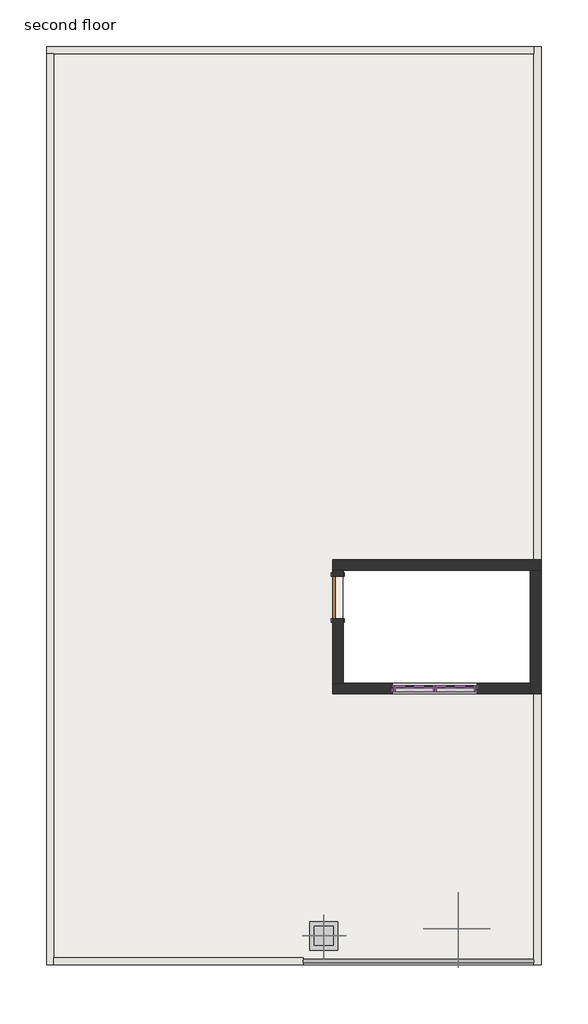
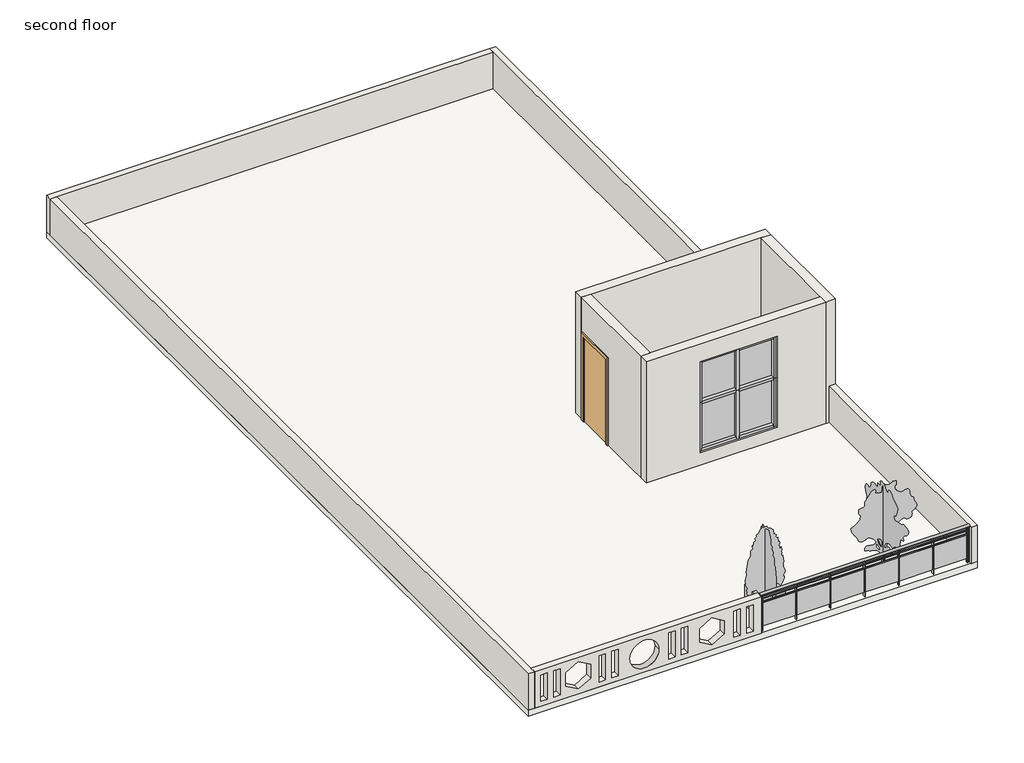
# One storey, incomplete: 12 members, 9 walls, 4 plates, 3 geographic elements, 1 door, 1 railing, 1 slab.
"""IFC4 building model written with IfcOpenShell, lengths in millimetres."""

from ifc_helpers import new_model, si_unit, point, frame, frame_2d, origin, place, context, project, spatial, polyline, circle_curve, ellipse_curve, trimmed, segment, composite_curve, outline, extrude, faceted_brep, transform, mapped, element, save
from ifc_brep_helpers import plane_surface, extruded_surface, advanced_brep
from components import single_flush_3_x7_0ca8825f, planter_2_x2_da431093, rpc_tree_conifer_chinese_juniper_7_1b9786cd, rpc_tree_deciduous_japanese_cherry_15_720dba75, member_c17f1be2, member_ad567e07, member_2b49869a, member_a715cb85, member_75074519, member_c4de40ee, system_panel_glazed_f4fd55f0, system_panel_glazed_231200ce

model = new_model("IFC4")

# Units and contexts
model_context = context("Model", 3, world=origin())
ifc_project = project(units=[si_unit("LENGTHUNIT", "METRE", prefix="MILLI")], contexts=[model_context])

# Site, building, storey
site = spatial("IfcSite", under=ifc_project)
building = spatial("IfcBuilding", under=site)
storey = spatial("IfcBuildingStorey", under=building, Name="second floor", Elevation=6400.8)

# Door
placement = place(None, origin())
single_flush_3_x7_shape = single_flush_3_x7_0ca8825f(model_context)
element("IfcDoor", 1, ObjectType="Single-Flush : 3'X7'", at=placement, inside=storey, context=model_context, shape_type="MappedRepresentation", body=[
    mapped(single_flush_3_x7_shape, transform((515.9585096, -1729.3523906, 6400.8), x_axis=(0.0, 1.0, 0.0), y_axis=(-1.0, 0.0, 0.0), z_axis=(0.0, 0.0, 1.0))),
])

# Geographic elements
planter_2_x2_shape = planter_2_x2_da431093(model_context)
element("IfcGeographicElement", 2, ObjectType="Planter : 2'x2'", at=placement, inside=storey, context=model_context, shape_type="MappedRepresentation", body=[
    mapped(planter_2_x2_shape, transform((211.1585096, -9031.8523906, 6400.8), x_axis=(1.0, 0.0, 0.0), y_axis=(0.0, 1.0, 0.0), z_axis=(0.0, 0.0, 1.0))),
])
rpc_tree_conifer_chinese_juniper_7_shape = rpc_tree_conifer_chinese_juniper_7_1b9786cd(model_context)
element("IfcGeographicElement", 3, ObjectType="RPC Tree - Conifer : Chinese Juniper - 7'", at=placement, inside=storey, context=model_context, shape_type="MappedRepresentation", body=[
    mapped(rpc_tree_conifer_chinese_juniper_7_shape, transform((210.9618385, -9031.8523906, 6400.8), x_axis=(1.0, 0.0, 0.0), y_axis=(0.0, 1.0, 0.0), z_axis=(0.0, 0.0, 1.0))),
])
rpc_tree_deciduous_japanese_cherry_15_shape = rpc_tree_deciduous_japanese_cherry_15_720dba75(model_context)
element("IfcGeographicElement", 4, ObjectType="RPC Tree - Deciduous : Japanese Cherry - 15'", at=placement, inside=storey, context=model_context, shape_type="MappedRepresentation", body=[
    mapped(rpc_tree_deciduous_japanese_cherry_15_shape, transform((3106.7585096, -8879.4523906, 6400.8), x_axis=(1.0, 0.0, 0.0), y_axis=(0.0, 1.0, 0.0), z_axis=(0.0, 0.0, 1.0))),
])

# Members
member_shape = member_c17f1be2(model_context)
element("IfcMember", 5, ObjectType="Rectangular Mullion : 2.5\" x 5\" rectangular", at=placement, inside=storey, context=model_context, shape_type="MappedRepresentation", body=[
    mapped(member_shape, transform((3456.0085096, -3697.8523906, 8991.6), x_axis=(0.0, 0.0, 1.0), y_axis=(0.0, -1.0, 0.0), z_axis=(1.0, 0.0, 0.0))),
])
element("IfcMember", 6, ObjectType="Rectangular Mullion : 2.5\" x 5\" rectangular", at=placement, inside=storey, context=model_context, shape_type="MappedRepresentation", body=[
    mapped(member_shape, transform((2573.3585096, -3697.8523906, 8991.6), x_axis=(0.0, 0.0, 1.0), y_axis=(0.0, -1.0, 0.0), z_axis=(1.0, 0.0, 0.0))),
])
element("IfcMember", 7, ObjectType="Rectangular Mullion : 2.5\" x 5\" rectangular", at=placement, inside=storey, context=model_context, shape_type="MappedRepresentation", body=[
    mapped(member_shape, transform((1754.2085096, -3697.8523906, 6705.6), x_axis=(0.0, 0.0, -1.0), y_axis=(0.0, -1.0, 0.0), z_axis=(-1.0, 0.0, 0.0))),
])
element("IfcMember", 8, ObjectType="Rectangular Mullion : 2.5\" x 5\" rectangular", at=placement, inside=storey, context=model_context, shape_type="MappedRepresentation", body=[
    mapped(member_shape, transform((2636.8585096, -3697.8523906, 6705.6), x_axis=(0.0, 0.0, -1.0), y_axis=(0.0, -1.0, 0.0), z_axis=(-1.0, 0.0, 0.0))),
])
member_2_shape = member_ad567e07(model_context)
element("IfcMember", 9, ObjectType="Rectangular Mullion : 2.5\" x 5\" rectangular", at=placement, inside=storey, context=model_context, shape_type="MappedRepresentation", body=[
    mapped(member_2_shape, transform((2573.3585096, -3697.8523906, 7924.8), x_axis=(0.0, 0.0, 1.0), y_axis=(0.0, -1.0, 0.0), z_axis=(1.0, 0.0, 0.0))),
])
element("IfcMember", 10, ObjectType="Rectangular Mullion : 2.5\" x 5\" rectangular", at=placement, inside=storey, context=model_context, shape_type="MappedRepresentation", body=[
    mapped(member_2_shape, transform((3456.0085096, -3697.8523906, 7924.8), x_axis=(0.0, 0.0, 1.0), y_axis=(0.0, -1.0, 0.0), z_axis=(1.0, 0.0, 0.0))),
])
member_3_shape = member_2b49869a(model_context)
element("IfcMember", 11, ObjectType="Rectangular Mullion : 2.5\" x 5\" rectangular", at=placement, inside=storey, context=model_context, shape_type="MappedRepresentation", body=[
    mapped(member_3_shape, transform((2605.1085096, -3697.8523906, 6705.6), x_axis=(1.0, 0.0, 0.0), y_axis=(0.0, -1.0, 0.0), z_axis=(0.0, 0.0, -1.0))),
])
member_4_shape = member_a715cb85(model_context)
element("IfcMember", 12, ObjectType="Rectangular Mullion : 2.5\" x 5\" rectangular", at=placement, inside=storey, context=model_context, shape_type="MappedRepresentation", body=[
    mapped(member_4_shape, transform((2605.1085096, -3697.8523906, 7924.8), x_axis=(1.0, 0.0, 0.0), y_axis=(0.0, -1.0, 0.0), z_axis=(0.0, 0.0, -1.0))),
])
member_5_shape = member_75074519(model_context)
element("IfcMember", 13, ObjectType="Rectangular Mullion : 2.5\" x 5\" rectangular", at=placement, inside=storey, context=model_context, shape_type="MappedRepresentation", body=[
    mapped(member_5_shape, transform((3519.5085096, -3697.8523906, 6705.6), x_axis=(1.0, 0.0, 0.0), y_axis=(0.0, -1.0, 0.0), z_axis=(0.0, 0.0, -1.0))),
])
member_6_shape = member_c4de40ee(model_context)
element("IfcMember", 14, ObjectType="Rectangular Mullion : 2.5\" x 5\" rectangular", at=placement, inside=storey, context=model_context, shape_type="MappedRepresentation", body=[
    mapped(member_6_shape, transform((1690.7085096, -3697.8523906, 8991.6), x_axis=(-1.0, 0.0, 0.0), y_axis=(0.0, -1.0, 0.0), z_axis=(0.0, 0.0, 1.0))),
])
element("IfcMember", 15, ObjectType="Rectangular Mullion : 2.5\" x 5\" rectangular", at=placement, inside=storey, context=model_context, shape_type="MappedRepresentation", body=[
    mapped(member_6_shape, transform((3519.5085096, -3697.8523906, 7924.8), x_axis=(1.0, 0.0, 0.0), y_axis=(0.0, -1.0, 0.0), z_axis=(0.0, 0.0, -1.0))),
])
element("IfcMember", 16, ObjectType="Rectangular Mullion : 2.5\" x 5\" rectangular", at=placement, inside=storey, context=model_context, shape_type="MappedRepresentation", body=[
    mapped(member_5_shape, transform((1690.7085096, -3697.8523906, 7924.8), x_axis=(-1.0, 0.0, 0.0), y_axis=(0.0, -1.0, 0.0), z_axis=(0.0, 0.0, 1.0))),
])

# Plates
system_panel_glazed_shape = system_panel_glazed_f4fd55f0(model_context)
element("IfcPlate", 17, ObjectType="System Panel : Glazed", at=placement, inside=storey, context=model_context, shape_type="MappedRepresentation", body=[
    mapped(system_panel_glazed_shape, transform((2163.7835096, -3697.8523906, 7956.55), x_axis=(1.0, 0.0, 0.0), y_axis=(0.0, 1.0, 0.0), z_axis=(0.0, 0.0, 1.0))),
])
element("IfcPlate", 18, ObjectType="System Panel : Glazed", at=placement, inside=storey, context=model_context, shape_type="MappedRepresentation", body=[
    mapped(system_panel_glazed_shape, transform((3046.4335096, -3697.8523906, 7956.55), x_axis=(1.0, 0.0, 0.0), y_axis=(0.0, 1.0, 0.0), z_axis=(0.0, 0.0, 1.0))),
])
system_panel_glazed_2_shape = system_panel_glazed_231200ce(model_context)
element("IfcPlate", 19, ObjectType="System Panel : Glazed", at=placement, inside=storey, context=model_context, shape_type="MappedRepresentation", body=[
    mapped(system_panel_glazed_2_shape, transform((2163.7835096, -3697.8523906, 6769.1), x_axis=(1.0, 0.0, 0.0), y_axis=(0.0, 1.0, 0.0), z_axis=(0.0, 0.0, 1.0))),
])
element("IfcPlate", 20, ObjectType="System Panel : Glazed", at=placement, inside=storey, context=model_context, shape_type="MappedRepresentation", body=[
    mapped(system_panel_glazed_2_shape, transform((3046.4335096, -3697.8523906, 6769.1), x_axis=(1.0, 0.0, 0.0), y_axis=(0.0, 1.0, 0.0), z_axis=(0.0, 0.0, 1.0))),
])

# Railing
element("IfcRailing", 21, ObjectType="Glass Panel - Bottom Fill", at=placement, inside=storey, context=model_context, shape_type="SolidModel", body=[
    advanced_brep(
    [(-234.9289904, -9539.8523906, 7315.2), (-234.9289904, -9616.0523906, 7315.2), (4745.0585096, -9539.8523906, 7315.2), (4745.0585096, -9616.0523906, 7315.2)],
    [
        (0, 1, ellipse_curve(frame((-234.9289904, -9577.9523906, 7315.2), z_axis=(-1.0, 0.0, 0.0), x_axis=(0.0, -1.0, 0.0)), 38.1, 28.575)),
        (1, 0, ellipse_curve(frame((-234.9289904, -9577.9523906, 7315.2), z_axis=(-1.0, 0.0, 0.0), x_axis=(0.0, -1.0, 0.0)), 38.1, 28.575)),
        (2, 3, ellipse_curve(frame((4745.0585096, -9577.9523906, 7315.2), z_axis=(1.0, 0.0, 0.0), x_axis=(0.0, -1.0, 0.0)), 38.1, 28.575)),
        (3, 2, ellipse_curve(frame((4745.0585096, -9577.9523906, 7315.2), z_axis=(1.0, 0.0, 0.0), x_axis=(0.0, -1.0, 0.0)), 38.1, 28.575)),
        (0, 2),
        (3, 1),
    ],
    [
        plane_surface(frame((-234.9289904, -9577.9523906, 7315.2), z_axis=(-1.0, 0.0, 0.0), x_axis=(0.0, 1.0, 0.0))),
        plane_surface(frame((4745.0585096, -9577.9523906, 7315.2), z_axis=(1.0, 0.0, 0.0), x_axis=(0.0, 1.0, 0.0))),
        extruded_surface(trimmed(ellipse_curve(frame((4745.0585096, -9577.9523906, 7315.2), z_axis=(-1.0, 0.0, 0.0), x_axis=(0.0, -1.0, 0.0)), 38.1, 28.575), [point((4745.0585096, -9539.8523906, 7315.2))], [point((4745.0585096, -9616.0523906, 7315.2))], True, "CARTESIAN"), (-4979.9875, 0.0, 0.0), 4979.9875),
        extruded_surface(trimmed(ellipse_curve(frame((4745.0585096, -9577.9523906, 7315.2), z_axis=(-1.0, 0.0, 0.0), x_axis=(0.0, -1.0, 0.0)), 38.1, 28.575), [point((4745.0585096, -9616.0523906, 7315.2))], [point((4745.0585096, -9539.8523906, 7315.2))], True, "CARTESIAN"), (-4979.9875, 0.0, 0.0), 4979.9875),
    ],
    [
        (0, [[1, 2]]),
        (1, [[3, 4]]),
        (2, [[-1, 5, -4, 6]]),
        (3, [[-2, -6, -3, -5]]),
    ],
),
    extrude(outline(polyline([(-234.9289904, -9590.6523906), (-234.9289904, -9565.2523906), (4745.0585096, -9565.2523906), (4745.0585096, -9590.6523906), (-234.9289904, -9590.6523906)])), frame((0.0, 0.0, 7200.9), z_axis=(0.0, 0.0, 1.0), x_axis=(1.0, 0.0, 0.0)), (0.0, 0.0, 1.0), 25.4),
    extrude(outline(polyline([(-234.9289904, -9590.6523906), (-234.9289904, -9565.2523906), (4745.0585096, -9565.2523906), (4745.0585096, -9590.6523906), (-234.9289904, -9590.6523906)])), frame((0.0, 0.0, 7099.3), z_axis=(0.0, 0.0, 1.0), x_axis=(1.0, 0.0, 0.0)), (0.0, 0.0, 1.0), 25.4),
    extrude(outline(polyline([(4687.1147596, -9603.3523906), (4687.1147596, -9552.5523906), (4699.8147596, -9552.5523906), (4699.8147596, -9603.3523906), (4687.1147596, -9603.3523906)])), frame((0.0, 0.0, 6400.8), z_axis=(0.0, 0.0, 1.0), x_axis=(1.0, 0.0, 0.0)), (0.0, 0.0, 1.0), 885.825),
    extrude(outline(polyline([(3880.6647596, -9571.4172336), (4693.4647596, -9571.4172336), (4693.4647596, -9577.7672336), (3880.6647596, -9577.7672336), (3880.6647596, -9571.4172336)])), frame((0.0, 0.0, 6502.4), z_axis=(0.0, 0.0, 1.0), x_axis=(1.0, 0.0, 0.0)), (0.0, 0.0, 1.0), 596.9),
    extrude(outline(polyline([(3874.3147596, -9603.3523906), (3874.3147596, -9552.5523906), (3887.0147596, -9552.5523906), (3887.0147596, -9603.3523906), (3874.3147596, -9603.3523906)])), frame((0.0, 0.0, 6400.8), z_axis=(0.0, 0.0, 1.0), x_axis=(1.0, 0.0, 0.0)), (0.0, 0.0, 1.0), 885.825),
    extrude(outline(polyline([(3067.8647596, -9571.4172336), (3880.6647596, -9571.4172336), (3880.6647596, -9577.7672336), (3067.8647596, -9577.7672336), (3067.8647596, -9571.4172336)])), frame((0.0, 0.0, 6502.4), z_axis=(0.0, 0.0, 1.0), x_axis=(1.0, 0.0, 0.0)), (0.0, 0.0, 1.0), 596.9),
    extrude(outline(polyline([(3061.5147596, -9603.3523906), (3061.5147596, -9552.5523906), (3074.2147596, -9552.5523906), (3074.2147596, -9603.3523906), (3061.5147596, -9603.3523906)])), frame((0.0, 0.0, 6400.8), z_axis=(0.0, 0.0, 1.0), x_axis=(1.0, 0.0, 0.0)), (0.0, 0.0, 1.0), 885.825),
    extrude(outline(polyline([(2255.0647596, -9571.4172336), (3067.8647596, -9571.4172336), (3067.8647596, -9577.7672336), (2255.0647596, -9577.7672336), (2255.0647596, -9571.4172336)])), frame((0.0, 0.0, 6502.4), z_axis=(0.0, 0.0, 1.0), x_axis=(1.0, 0.0, 0.0)), (0.0, 0.0, 1.0), 596.9),
    extrude(outline(polyline([(2248.7147596, -9603.3523906), (2248.7147596, -9552.5523906), (2261.4147596, -9552.5523906), (2261.4147596, -9603.3523906), (2248.7147596, -9603.3523906)])), frame((0.0, 0.0, 6400.8), z_axis=(0.0, 0.0, 1.0), x_axis=(1.0, 0.0, 0.0)), (0.0, 0.0, 1.0), 885.825),
    extrude(outline(polyline([(1442.2647596, -9571.4172336), (2255.0647596, -9571.4172336), (2255.0647596, -9577.7672336), (1442.2647596, -9577.7672336), (1442.2647596, -9571.4172336)])), frame((0.0, 0.0, 6502.4), z_axis=(0.0, 0.0, 1.0), x_axis=(1.0, 0.0, 0.0)), (0.0, 0.0, 1.0), 596.9),
    extrude(outline(polyline([(1435.9147596, -9603.3523906), (1435.9147596, -9552.5523906), (1448.6147596, -9552.5523906), (1448.6147596, -9603.3523906), (1435.9147596, -9603.3523906)])), frame((0.0, 0.0, 6400.8), z_axis=(0.0, 0.0, 1.0), x_axis=(1.0, 0.0, 0.0)), (0.0, 0.0, 1.0), 885.825),
    extrude(outline(polyline([(629.4647596, -9571.4172336), (1442.2647596, -9571.4172336), (1442.2647596, -9577.7672336), (629.4647596, -9577.7672336), (629.4647596, -9571.4172336)])), frame((0.0, 0.0, 6502.4), z_axis=(0.0, 0.0, 1.0), x_axis=(1.0, 0.0, 0.0)), (0.0, 0.0, 1.0), 596.9),
    extrude(outline(polyline([(623.1147596, -9603.3523906), (623.1147596, -9552.5523906), (635.8147596, -9552.5523906), (635.8147596, -9603.3523906), (623.1147596, -9603.3523906)])), frame((0.0, 0.0, 6400.8), z_axis=(0.0, 0.0, 1.0), x_axis=(1.0, 0.0, 0.0)), (0.0, 0.0, 1.0), 885.825),
    extrude(outline(polyline([(-183.3352404, -9571.4172336), (629.4647596, -9571.4172336), (629.4647596, -9577.7672336), (-183.3352404, -9577.7672336), (-183.3352404, -9571.4172336)])), frame((0.0, 0.0, 6502.4), z_axis=(0.0, 0.0, 1.0), x_axis=(1.0, 0.0, 0.0)), (0.0, 0.0, 1.0), 596.9),
    extrude(outline(polyline([(-189.6852404, -9603.3523906), (-189.6852404, -9552.5523906), (-176.9852404, -9552.5523906), (-176.9852404, -9603.3523906), (-189.6852404, -9603.3523906)])), frame((0.0, 0.0, 6400.8), z_axis=(0.0, 0.0, 1.0), x_axis=(1.0, 0.0, 0.0)), (0.0, 0.0, 1.0), 885.825),
    extrude(outline(polyline([(4732.3585096, -9587.4773906), (4732.3585096, -9568.4273906), (4751.4085096, -9568.4273906), (4751.4085096, -9587.4773906), (4732.3585096, -9587.4773906)])), frame((0.0, 0.0, 6400.8), z_axis=(0.0, 0.0, 1.0), x_axis=(1.0, 0.0, 0.0)), (0.0, 0.0, 1.0), 885.825),
    extrude(outline(polyline([(-241.2789904, -9587.4773906), (-241.2789904, -9568.4273906), (-222.2289904, -9568.4273906), (-222.2289904, -9587.4773906), (-241.2789904, -9587.4773906)])), frame((0.0, 0.0, 6400.8), z_axis=(0.0, 0.0, 1.0), x_axis=(1.0, 0.0, 0.0)), (0.0, 0.0, 1.0), 885.825),
])

# Slab
element("IfcSlab", 22, ObjectType="6\"", at=placement, inside=storey, context=model_context, shape_type="SweptSolid", body=[
    extrude(outline(polyline([(4897.4585096, 10157.8476094), (4897.4585096, -9654.1523906), (-5772.1289904, -9654.1523906), (-5772.1289904, 10157.8476094), (4897.4585096, 10157.8476094)]), holes=[polyline([(4668.8585096, -1145.1523906), (630.2585096, -1145.1523906), (630.2585096, -3583.5523906), (4668.8585096, -3583.5523906), (4668.8585096, -1145.1523906)])]), frame((0.0, 0.0, 6248.4), z_axis=(0.0, 0.0, 1.0), x_axis=(1.0, 0.0, 0.0)), (0.0, 0.0, 1.0), 152.4),
])

# Walls
element("IfcWall", 23, ObjectType="6\"", at=placement, inside=storey, context=model_context, shape_type="SweptSolid", body=[
    extrude(outline(polyline([(4897.4585096, -3812.1523906), (4897.4585096, -9654.1523906), (4745.0585096, -9654.1523906), (4745.0585096, -3812.1523906), (4897.4585096, -3812.1523906)])), frame((0.0, 0.0, 6400.8), z_axis=(0.0, 0.0, 1.0), x_axis=(1.0, 0.0, 0.0)), (0.0, 0.0, 1.0), 914.4),
])
element("IfcWall", 24, ObjectType="6\"", at=placement, inside=storey, context=model_context, shape_type="Brep", body=[
    faceted_brep([(4897.4585096, -916.5523906, 6400.8), (4897.4585096, 10157.8476094, 6400.8), (4897.4585096, 10157.8476094, 7315.2), (4897.4585096, -916.5523906, 7315.2), (4745.0585096, -916.5523906, 6400.8), (4745.0585096, -916.5523906, 7315.2), (4745.0585096, 10005.4476094, 7315.2), (4745.0585096, 10157.8476094, 7315.2), (4745.0585096, 10157.8476094, 6400.8), (4745.0585096, 10005.4476094, 6400.8)], [[[0, 1, 2, 3]], [[4, 5, 6, 7, 8, 9]], [[1, 0, 4, 9, 8]], [[3, 2, 7, 6, 5]], [[0, 3, 5, 4]], [[2, 1, 8, 7]]]),
])
element("IfcWall", 25, ObjectType="6\"", at=placement, inside=storey, context=model_context, shape_type="Brep", body=[
    faceted_brep([(4745.0585096, 10157.8476094, 6400.8), (-5772.1289904, 10157.8476094, 6400.8), (-5772.1289904, 10157.8476094, 7315.2), (4745.0585096, 10157.8476094, 7315.2), (4745.0585096, 10005.4476094, 6400.8), (4745.0585096, 10005.4476094, 7315.2), (-5619.7289904, 10005.4476094, 7315.2), (-5772.1289904, 10005.4476094, 7315.2), (-5772.1289904, 10005.4476094, 6400.8), (-5619.7289904, 10005.4476094, 6400.8)], [[[0, 1, 2, 3]], [[4, 5, 6, 7, 8, 9]], [[1, 0, 4, 9, 8]], [[3, 2, 7, 6, 5]], [[0, 3, 5, 4]], [[2, 1, 8, 7]]]),
])
element("IfcWall", 26, ObjectType="6\"", at=placement, inside=storey, context=model_context, shape_type="Brep", body=[
    faceted_brep([(-5772.1289904, 10005.4476094, 6400.8), (-5772.1289904, -9654.1523906, 6400.8), (-5772.1289904, -9654.1523906, 7315.2), (-5772.1289904, 10005.4476094, 7315.2), (-5619.7289904, 10005.4476094, 6400.8), (-5619.7289904, 10005.4476094, 7315.2), (-5619.7289904, -9501.7523906, 7315.2), (-5619.7289904, -9654.1523906, 7315.2), (-5619.7289904, -9654.1523906, 6400.8), (-5619.7289904, -9501.7523906, 6400.8)], [[[0, 1, 2, 3]], [[4, 5, 6, 7, 8, 9]], [[1, 0, 4, 9, 8]], [[3, 2, 7, 6, 5]], [[0, 3, 5, 4]], [[2, 1, 8, 7]]]),
])
element("IfcWall", 27, ObjectType="6\"", at=placement, inside=storey, context=model_context, shape_type="SweptSolid", body=[
    extrude(outline(polyline([(6400.8, -5619.7289904), (6400.8, -234.9289904), (7315.2, -234.9289904), (7315.2, -5619.7289904), (6400.8, -5619.7289904)]), holes=[polyline([(7179.5349677, -5320.3553103), (6519.1349677, -5320.3553103), (6519.1349677, -5472.7553103), (7179.5349677, -5472.7553103), (7179.5349677, -5320.3553103)]), polyline([(7179.5349677, -5015.5553103), (6519.1349677, -5015.5553103), (6519.1349677, -5167.9553103), (7179.5349677, -5167.9553103), (7179.5349677, -5015.5553103)]), polyline([(7179.5349677, -3936.0553103), (6519.1349677, -3936.0553103), (6519.1349677, -4088.4553103), (7179.5349677, -4088.4553103), (7179.5349677, -3936.0553103)]), polyline([(7179.5349677, -3631.2553103), (6519.1349677, -3631.2553103), (6519.1349677, -3783.6553103), (7179.5349677, -3783.6553103), (7179.5349677, -3631.2553103)]), polyline([(7179.5349677, -735.6553103), (6519.1349677, -735.6553103), (6519.1349677, -888.0553103), (7179.5349677, -888.0553103), (7179.5349677, -735.6553103)]), polyline([(7179.5349677, -430.8553103), (6519.1349677, -430.8553103), (6519.1349677, -583.2553103), (7179.5349677, -583.2553103), (7179.5349677, -430.8553103)]), polyline([(7179.5349677, -2285.0553103), (6519.1349677, -2285.0553103), (6519.1349677, -2437.4553103), (7179.5349677, -2437.4553103), (7179.5349677, -2285.0553103)]), polyline([(7179.5349677, -1980.2553103), (6519.1349677, -1980.2553103), (6519.1349677, -2132.6553103), (7179.5349677, -2132.6553103), (7179.5349677, -1980.2553103)]), polyline([(6689.9534558, -4879.7672744), (7031.590432, -4879.7672744), (7202.4089202, -4583.9009741), (7031.590432, -4288.0346737), (6689.9534558, -4288.0346737), (6519.1349677, -4583.9009741), (6689.9534558, -4879.7672744)]), composite_curve([segment(trimmed(circle_curve(frame_2d((6843.5450551, -3013.498529)), 345.2300042), [point((6843.5450551, -2668.2685248))], [point((6843.5450551, -3358.7285332))], True, "CARTESIAN"), True, "CONTINUOUS"), segment(trimmed(circle_curve(frame_2d((6843.5450551, -3013.498529)), 345.2300042), [point((6843.5450551, -3358.7285332))], [point((6843.5450551, -2668.2685248))], True, "CARTESIAN"), True, "CONTINUOUS")], self_intersect=False), polyline([(6687.2184638, -1699.6372677), (7023.3854561, -1699.6372677), (7191.4689522, -1408.5081124), (7023.3854561, -1117.3789572), (6687.2184638, -1117.3789572), (6519.1349677, -1408.5081124), (6687.2184638, -1699.6372677)])]), frame((0.0, -9654.1523906, 0.0), z_axis=(0.0, 1.0, 0.0), x_axis=(0.0, 0.0, 1.0)), (0.0, 0.0, 1.0), 152.4),
])
element("IfcWall", 28, ObjectType="9\" 2", at=placement, inside=storey, context=model_context, shape_type="Brep", body=[
    faceted_brep([(401.6585096, -1145.1523906, 6400.8), (630.2585096, -1145.1523906, 6400.8), (4668.8585096, -1145.1523906, 6400.8), (4897.4585096, -1145.1523906, 6400.8), (4897.4585096, -1145.1523906, 9448.8), (4668.8585096, -1145.1523906, 9448.8), (630.2585096, -1145.1523906, 9448.8), (401.6585096, -1145.1523906, 9448.8), (401.6585096, -916.5523906, 6400.8), (401.6585096, -916.5523906, 9448.8), (4897.4585096, -916.5523906, 9448.8), (4897.4585096, -916.5523906, 7315.2), (4897.4585096, -916.5523906, 6400.8), (4745.0585096, -916.5523906, 6400.8)], [[[0, 1, 2, 3, 4, 5, 6, 7]], [[8, 9, 10, 11, 12, 13]], [[3, 2, 1, 0, 8, 13, 12]], [[7, 6, 5, 4, 10, 9]], [[0, 7, 9, 8]], [[3, 12, 11, 10, 4]]]),
])
element("IfcWall", 29, ObjectType="9\" 2", at=placement, inside=storey, context=model_context, shape_type="Brep", body=[
    faceted_brep([(4668.8585096, -1145.1523906, 9448.8), (4668.8585096, -1145.1523906, 6400.8), (4668.8585096, -3583.5523906, 6400.8), (4668.8585096, -3812.1523906, 6400.8), (4668.8585096, -3812.1523906, 9448.8), (4668.8585096, -3583.5523906, 9448.8), (4897.4585096, -1145.1523906, 6400.8), (4897.4585096, -1145.1523906, 9448.8), (4897.4585096, -3812.1523906, 9448.8), (4897.4585096, -3812.1523906, 7315.2), (4897.4585096, -3812.1523906, 6400.8), (4745.0585096, -3812.1523906, 6400.8)], [[[0, 1, 2, 3, 4, 5]], [[6, 7, 8, 9, 10]], [[3, 2, 1, 6, 10, 11]], [[0, 5, 4, 8, 7]], [[3, 11, 10, 9, 8, 4]], [[0, 7, 6, 1]]]),
])
element("IfcWall", 30, ObjectType="9\" 2", at=placement, inside=storey, context=model_context, shape_type="Brep", body=[
    faceted_brep([(4668.8585096, -3583.5523906, 6400.8), (630.2585096, -3583.5523906, 6400.8), (401.6585096, -3583.5523906, 6400.8), (401.6585096, -3583.5523906, 9448.8), (630.2585096, -3583.5523906, 9448.8), (4668.8585096, -3583.5523906, 9448.8), (1690.7085096, -3583.5523906, 8991.6), (1690.7085096, -3583.5523906, 6705.6), (3519.5085096, -3583.5523906, 6705.6), (3519.5085096, -3583.5523906, 8991.6), (401.6585096, -3812.1523906, 6400.8), (4668.8585096, -3812.1523906, 6400.8), (4668.8585096, -3812.1523906, 9448.8), (401.6585096, -3812.1523906, 9448.8), (1690.7085096, -3812.1523906, 6705.6), (1690.7085096, -3812.1523906, 8991.6), (3519.5085096, -3812.1523906, 8991.6), (3519.5085096, -3812.1523906, 6705.6)], [[[0, 1, 2, 3, 4, 5], [6, 7, 8, 9]], [[10, 11, 12, 13], [14, 15, 16, 17]], [[2, 1, 0, 11, 10]], [[5, 4, 3, 13, 12]], [[3, 2, 10, 13]], [[14, 7, 6, 15]], [[15, 6, 9, 16]], [[16, 9, 8, 17]], [[7, 14, 17, 8]], [[5, 12, 11, 0]]]),
])
element("IfcWall", 31, ObjectType="9\" 2", at=placement, inside=storey, context=model_context, shape_type="SweptSolid", body=[
    extrude(outline(polyline([(-1145.1523906, 6400.8), (-1272.1523906, 6400.8), (-1272.1523906, 8534.4), (-2186.5523906, 8534.4), (-2186.5523906, 6400.8), (-3583.5523906, 6400.8), (-3583.5523906, 9448.8), (-1145.1523906, 9448.8), (-1145.1523906, 6400.8)])), frame((401.6585096, 0.0, 0.0), z_axis=(1.0, 0.0, 0.0), x_axis=(0.0, 1.0, 0.0)), (0.0, 0.0, 1.0), 228.6),
])

save(model, "model.ifc")

# Revit data of these elements
# Type "Single-Flush : 3'X7'"
#   Type Mark = "8"
#   Construction Type Id = "MDOOR"
#   Assembly Code = "C1020"
#   Analytic Construction = "Metal"
#   Thickness = 0' - 2"
#   Heat Transfer Coefficient (U) = 0.651978 BTU/(h·ft²·°F)
#   Height = 7' - 0"
#   Trim Projection Ext = 0' - 1"
#   Trim Projection Int = 0' - 1"
#   Trim Width = 0' - 3"
#   Width = 3' - 0"
#   Define Thermal Properties by = 1
#   Door Material = Door - Panel
#   Frame Material = Door - Frame
#   Visual Light Transmittance = 0
#   Solar Heat Gain Coefficient = 0
#   Function = (empty or 0)
#   Wall Closure = (empty or 0)
# Type "Planter : 2'x2'"
#   Depth = 2' - 0"
#   Height = 2' - 0"
#   Width = 2' - 0"
#   Material = Concrete, Precast
# Type "RPC Tree - Conifer : Chinese Juniper - 7'"
#   built-in parameter 1005198 = "{2, 15},{39, RPC-16-FUM3-UUQ0-UBF0-N000-ST1L-LVER-AU},{1, 0},{1, 0},{2, 35},{1, 8},{5, Color},{1, 0},{1, 0},{3, 0.8},{3, 0.8},{3, 0.8},{1, 8},{7, BBoxMin},{1, 0},{1, 0},{1, 0},{1, 0},{1, 0},{1, 8},{7, BBoxMax},{1, 0},{1, 0},{1, 0},{1, 0},{1, 0},{2, 11},{9, RPCTypeId},{1, 0},{1, 0},{39, RPC-16-FUM3-UUQ0-UBF0-N000-ST1L-LVER-AU},{1, 6},{14, RPCPlantHeight},{1, 0},{1, 0},{1, 7},{2, 11},{7, keyword},{1, 0},{1, 0},{96, :Geometry:RPC:Chinese Juniper:juniperus chinensis:chinese:juniper:cupressaceae:conifer:evergreen},{2, 11},{8, category},{1, 0},{1, 0},{16, :Trees [General]},{2, 11},{12, LocalizedUID},{1, 0},{1, 0},{15, Chinese Juniper},{2, 14},{6, Height},{1, 0},{1, 0},{1, 7},{1, 2},{16, Cast Reflections},{1, 0},{1, 0},{1, 0},{1, 2},{12, Cast Shadows},{1, 0},{1, 0},{1, 1},{1, 2},{9, Lock View},{1, 0},{1, 0},{1, 0},{1, 4},{5, ViewC},{1, 0},{1, 0},{1, 0},{2, 11},{20, AdvancedUIDefinition},{1, 0},{1, 0},{0, },{2, 11},{10, AssetLibID},{1, 0},{1, 0},{36, 4D3F6E72-3F99-4203-98E9-AF80B3C7A7A4},{2, 11},{10, BaseSchema},{1, 0},{1, 0},{9, RPCSchema},{2, 11},{12, ExchangeGUID},{1, 0},{1, 0},{0, },{1, 2},{6, Hidden},{1, 0},{1, 0},{1, 0},{1, 4},{11, RPCCategory},{1, 0},{1, 0},{1, 0},{2, 11},{8, RPCImage},{1, 0},{1, 0},{0, },{1, 4},{13, SchemaVersion},{1, 0},{1, 0},{1, 4},{2, 11},{12, UIDefinition},{1, 0},{1, 0},{0, },{2, 11},{6, UIName},{1, 0},{1, 0},{39, RPC-16-FUM3-UUQ0-UBF0-N000-ST1L-LVER-AU},{2, 11},{11, VersionGUID},{1, 0},{1, 0},{9, RPCSchema},{2, 11},{9, assettype},{1, 0},{1, 0},{11, RPCGeometry},{2, 11},{11, description},{1, 0},{1, 0},{0, },{2, 11},{9, localname},{1, 0},{1, 0},{3, RPC},{2, 11},{9, localtype},{1, 0},{1, 0},{3, RPC},{1, 4},{8, revision},{1, 0},{1, 0},{1, 1},{2, 11},{9, thumbnail},{1, 0},{1, 0},{0, },{1, 4},{7, version},{1, 0},{1, 0},{1, 1},{1, 2},{20, RPC_Cast Reflections},{1, 0},{1, 0},{1, 1},{1, 2},{16, RPC_Cast Shadows},{1, 0},{1, 0},{1, 1},{1, 2},{13, RPC_Lock View},{1, 0},{1, 0},{1, 0},{1, 4},{9, RPC_ViewC},{1, 0},{1, 0},{1, 0},{21, assetlibrary_base.fbx},{1, 5},"
#   built-in parameter 1005195 = "RPC-16-FUM3-UUQ0-UBF0-N000-ST1L-LVER-AU"
#   Type Comments = "Chinese Juniper"
#   Assembly Code = "G2050500"
#   Height = 7' - 0"
#   Description = (empty or 0)
#   Default Elevation = 0
# Type "RPC Tree - Deciduous : Japanese Cherry - 15'"
#   built-in parameter 1005198 = "{2, 15},{39, RPC-16-FXGW-2MQ0-PN7K-A000-ST1L-LVER-AU},{1, 0},{1, 0},{2, 35},{1, 8},{5, Color},{1, 0},{1, 0},{3, 0.8},{3, 0.8},{3, 0.8},{1, 8},{7, BBoxMin},{1, 0},{1, 0},{1, 0},{1, 0},{1, 0},{1, 8},{7, BBoxMax},{1, 0},{1, 0},{1, 0},{1, 0},{1, 0},{2, 11},{9, RPCTypeId},{1, 0},{1, 0},{39, RPC-16-FXGW-2MQ0-PN7K-A000-ST1L-LVER-AU},{1, 6},{14, RPCPlantHeight},{1, 0},{1, 0},{2, 15},{2, 11},{7, keyword},{1, 0},{1, 0},{207, :Geometry:RPC:Japanese Flowering Cherry:Prunus serrulata Lindl:A landscape tree:valued for its abundant showy flowers; native to China and Japan.  Hardy only in the mildest parts of Canada and farther south.},{2, 11},{8, category},{1, 0},{1, 0},{16, :Trees [General]},{2, 11},{12, LocalizedUID},{1, 0},{1, 0},{25, Japanese Flowering Cherry},{2, 14},{6, Height},{1, 0},{1, 0},{2, 15},{1, 2},{16, Cast Reflections},{1, 0},{1, 0},{1, 0},{1, 2},{12, Cast Shadows},{1, 0},{1, 0},{1, 1},{1, 2},{9, Lock View},{1, 0},{1, 0},{1, 0},{1, 4},{5, ViewC},{1, 0},{1, 0},{1, 0},{2, 11},{20, AdvancedUIDefinition},{1, 0},{1, 0},{0, },{2, 11},{10, AssetLibID},{1, 0},{1, 0},{36, 4D3F6E72-3F99-4203-98E9-AF80B3C7A7A4},{2, 11},{10, BaseSchema},{1, 0},{1, 0},{9, RPCSchema},{2, 11},{12, ExchangeGUID},{1, 0},{1, 0},{0, },{1, 2},{6, Hidden},{1, 0},{1, 0},{1, 0},{1, 4},{11, RPCCategory},{1, 0},{1, 0},{1, 0},{2, 11},{8, RPCImage},{1, 0},{1, 0},{0, },{1, 4},{13, SchemaVersion},{1, 0},{1, 0},{1, 4},{2, 11},{12, UIDefinition},{1, 0},{1, 0},{0, },{2, 11},{6, UIName},{1, 0},{1, 0},{39, RPC-16-FXGW-2MQ0-PN7K-A000-ST1L-LVER-AU},{2, 11},{11, VersionGUID},{1, 0},{1, 0},{9, RPCSchema},{2, 11},{9, assettype},{1, 0},{1, 0},{11, RPCGeometry},{2, 11},{11, description},{1, 0},{1, 0},{0, },{2, 11},{9, localname},{1, 0},{1, 0},{3, RPC},{2, 11},{9, localtype},{1, 0},{1, 0},{3, RPC},{1, 4},{8, revision},{1, 0},{1, 0},{1, 1},{2, 11},{9, thumbnail},{1, 0},{1, 0},{0, },{1, 4},{7, version},{1, 0},{1, 0},{1, 1},{1, 2},{20, RPC_Cast Reflections},{1, 0},{1, 0},{1, 1},{1, 2},{16, RPC_Cast Shadows},{1, 0},{1, 0},{1, 1},{1, 2},{13, RPC_Lock View},{1, 0},{1, 0},{1, 0},{1, 4},{9, RPC_ViewC},{1, 0},{1, 0},{1, 0},{21, assetlibrary_base.fbx},{1, 5},"
#   built-in parameter 1005195 = "RPC-16-FXGW-2MQ0-PN7K-A000-ST1L-LVER-AU"
#   Type Comments = "Japanese Cherry"
#   Assembly Code = "G2050500"
#   Height = 7' - 0"
#   Default Elevation = 0
# Type "Rectangular Mullion : 2.5\" x 5\" rectangular"
#   built-in parameter 1007304 = 0.416667 (stored number, unit not read)
#   built-in parameter 1007301 = 0.104167 (stored number, unit not read)
#   built-in parameter 1007300 = 0.104167 (stored number, unit not read)
# Type "System Panel : Glazed"
#   Construction Type Id = "GSP4R"
#   Analytic Construction = "1/8 in Pilkington single glazing"
#   Visual Light Transmittance = 0.9
#   Solar Heat Gain Coefficient = 0.86
#   Heat Transfer Coefficient (U) = 1.18115 BTU/(h·ft²·°F)
#   Define Thermal Properties by = 1
# Type "Glass Panel - Bottom Fill"
#   Assembly Code = "C2010400"
#   built-in parameter 1008612 = 0.0416667 (stored number, unit not read)
#   built-in parameter 1008611 = 0.0416667 (stored number, unit not read)
#   built-in parameter 1008609 = 0.333333 (stored number, unit not read)
#   built-in parameter 1008604 = 0.166667 (stored number, unit not read)
#   built-in parameter 1008603 = 0.166667 (stored number, unit not read)
#   Railing Height = 3' - 0"
#   built-in parameter 1008630 = 2
#   built-in parameter 1008610 = 2
#   built-in parameter 1008618 = Baluster - Square : 3/4"
# Type "6\""
#   Assembly Code = "B1010"
#   Function = 0
#   Layers, outside or top first: 0' - 6" no material (function 1)
# Type "6\""
#   Assembly Code = "B2010"
#   Layers, outside or top first: 0' - 6" "wall 2" (function 1)
# Type "9\" 2"
#   Assembly Code = "B2010"
#   Layers, outside or top first: 0' - 9" "wall" (function 1)
# Element 1 (IfcDoor, "Single-Flush : 3'X7'")
#   Phase Created = New Construction
#   Materials on its faces: "Door - Frame", "Door - Panel"
# Element 2 (IfcGeographicElement, "Planter : 2'x2'")
#   Phase Created = New Construction
#   Materials on its faces: "Concrete, Precast"
# Element 3 (IfcGeographicElement, "RPC Tree - Conifer : Chinese Juniper - 7'")
#   Phase Created = New Construction
# Element 4 (IfcGeographicElement, "RPC Tree - Deciduous : Japanese Cherry - 15'")
#   Phase Created = New Construction
# Elements 5, 6, 7, 8, 9, 10, 11, 12, 13, 14, 15, 16 (IfcMember, "Rectangular Mullion : 2.5\" x 5\" rectangular")
#   Phase Created = New Construction
#   Materials on its faces: "Aluminum"
# Elements 17, 18, 19, 20 (IfcPlate, "System Panel : Glazed")
#   Phase Created = New Construction
#   Materials on its faces: "Glass"
# Element 21 (IfcRailing, "Glass Panel - Bottom Fill")
#   Phase Created = New Construction
#   Materials on its faces: "Glass"
# Element 22 (IfcSlab, "6\"")
#   Height Offset From Level = 0' - 0"
#   Phase Created = New Construction
#   Materials on its faces: "Default Floor", "wood 1", "wall 2"
# Elements 23, 24, 25, 26, 27 (IfcWall, "6\"")
#   Top Offset = -0' - 6"
#   Base Offset = 0' - 0"
#   Unconnected Height = 3' - 0"
#   wall height = 3' - 0"
#   Phase Created = New Construction
#   Base Constraint = second floor
#   Materials on its faces: "wall 2"
# Elements 28, 29, 30 (IfcWall, "9\" 2")
#   Top Offset = -0' - 6"
#   Base Offset = 0' - 0"
#   wall height = 10' - 0"
#   Phase Created = New Construction
#   Base Constraint = second floor
#   Top Constraint = roof
#   Materials on its faces: "wall", "wall 1"
# Element 31 (IfcWall, "9\" 2")
#   Top Offset = -0' - 6"
#   Base Offset = 0' - 0"
#   wall height = 10' - 0"
#   Phase Created = New Construction
#   Base Constraint = second floor
#   Top Constraint = roof
#   Materials on its faces: "wall"
# Materials
#   "Door - Panel": class "Wood", colour RGB 210 159 95, transparency 0, Cost = 0
#   "Door - Frame": colour RGB 118 70 51, transparency 0, Cost = 0
#   "Concrete, Precast": class "Concrete", colour RGB 198 187 187, transparency 0, Description = "Precast concrete", Cost = 0
#   "wall 2": class "Generic", colour RGB 34 30 27, transparency 0, Cost = 0
#   "wall": class "Generic", colour RGB 93 108 103, transparency 0, Cost = 0
#   "Aluminum": class "Metal", colour RGB 247 247 247, transparency 0, Description = "Aluminum 6061", Cost = 0
#   "Glass": class "Glass", colour RGB 0 128 192, transparency 0.75, Description = "Soda Lime Glass", Cost = 0
#   "Default Floor": colour RGB 128 128 128, transparency 0, Cost = 0
#   "wood 1": class "Generic", colour RGB 51 32 15, transparency 0, Cost = 0
#   "wall 1": class "Generic", colour RGB 133 142 137, transparency 0, Cost = 0
